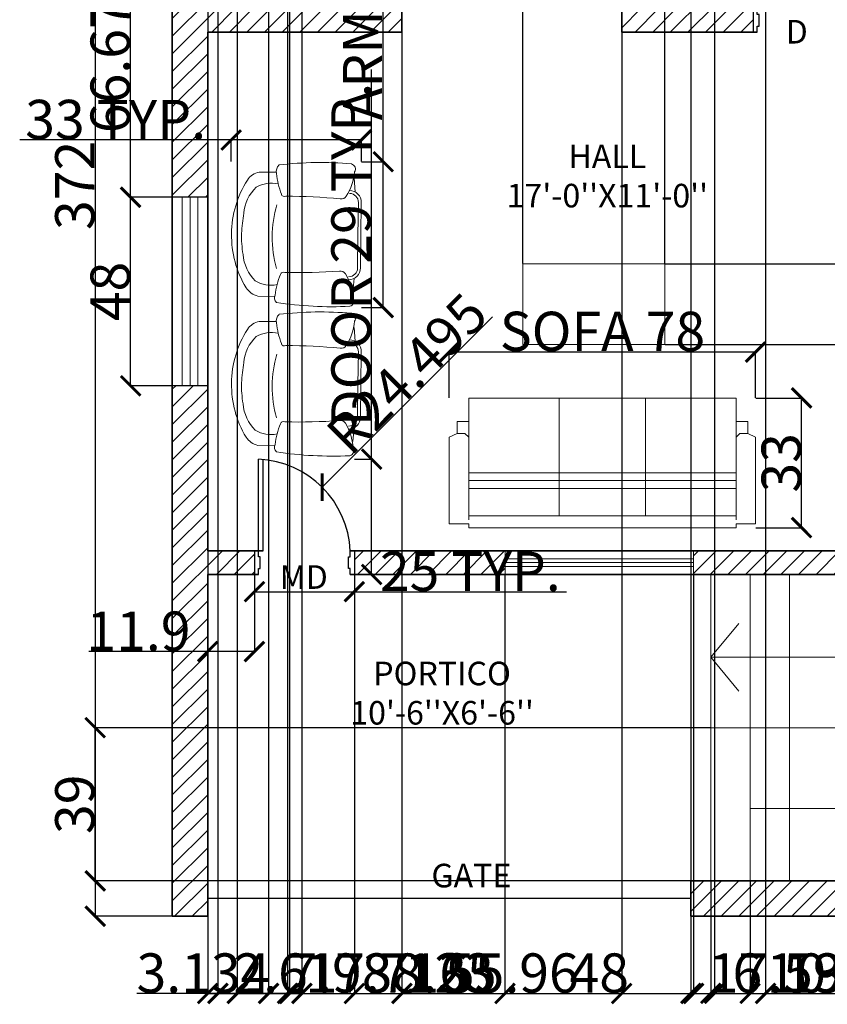
# Model space of a CAD drawing. Units: inches. Extents: x 90933 to 91345, y 21207 to 21646.
# Tile 1 of 4: x 90989 to 91195, y 21207 to 21458. Entities that reach past the tile are written whole.
import ezdxf

# ---------------------------------------------------------------- set-up
doc = ezdxf.new("R2010")
doc.units = ezdxf.units.IN
for name, color, linetype, lineweight in [('A-ANNO-DIMS', 2, 'Continuous', 18), ('A-ANNO-TEXT', 7, 'Continuous', 18), ('A-AREA-IDEN', 7, 'Continuous', 25), ('A-WALL-PATT', 8, 'Continuous', 13), ('B-FURNITURE', 9, 'Continuous', 18), ('Doors', 34, 'Continuous', 25), ('Steps', 50, 'Continuous', 18), ('Walls', 7, 'Continuous', 35), ('Windows', 140, 'Continuous', 18)]:
    doc.layers.add(name, color=color, linetype=linetype, lineweight=lineweight)
doc.styles.get("Standard").update_dxf_attribs({"font": 'arial.ttf'})
doc.dimstyles.get("Standard").update_dxf_attribs({"dimtxt": 10, "dimasz": 5, "dimexe": 0.18, "dimexo": 0.0625, "dimgap": 0.09, "dimtad": 1, "dimdec": 1, "dimzin": 0, "dimdsep": 46, "dimlunit": 4, "dimtxsty": 'Standard', "dimblk": 'ARCHTICK', "dimcen": 0.09, "dimadec": 0, "dimazin": 0, "dimtfac": 1, "dimtdec": 1, "dimtofl": 0, "dimtmove": 0, "dimatfit": 3, "dimldrblk": 'NONE', "dimfxl": 1, "dimtolj": 1, "dimtzin": 0, "dimarcsym": 0})

# ---------------------------------------------------------------- blocks, each defined once
blk = doc.blocks.new('12PCOU13')
at = {"color": 0, "linetype": 'ByBlock'}
for p, q in [((24, 37), (24, 35)), ((23, 34), (2, 34)), ((3, -34), (3, 34)), ((10, 34), (10, -34)), ((12, 34), (12, -34)), ((14, 34), (14, -34)), ((24, 35), (23, 34)), ((27, 34), (23, 34)), ((33, 11), (3, 11)), ((33, -11), (3, -11)), ((23, -34), (2, -34)), ((27, -34), (23, -34)), ((24, -35), (23, -34)), ((24, -37), (24, -35))]:
    blk.add_line(p, q, dxfattribs=at)
blk.add_lwpolyline([(1, -39), (1, -34), (0, -34), (0, 34), (1, 34), (1, 39), (23, 39), (24, 37), (27, 37), (27, 34), (33, 34), (33, -34), (27, -34), (27, -37), (24, -37), (23, -39)], close=True, dxfattribs=at)
blk = doc.blocks.new('A$C198557BC')
for p, q in [((-0.4117, 0.5807), (-0.4097, 0.6946)), ((0.4248, 0.5712), (0.4254, 0.6851)), ((-0.2994, 0.0834), (-0.2994, 0.0852)), ((0.3012, 0.0766), (0.3012, 0.0783)), ((-0.2905, 0.0459), (-0.3822, 0.0549)), ((0, 0), (-0.2203, 0.0025)), ((0.0002, 0.02), (-0.2201, 0.0225)), ((0, 0), (0.2203, -0.0025)), ((0.0002, 0.02), (0.2205, 0.0175)), ((0.2915, 0.0393), (0.3834, 0.0462))]:
    blk.add_line(p, q)
for centre, radius, start, end in [((-0.0029, 0.1962), 0.6755, 88.91413, 121.26982), ((0.0052, 0.1888), 0.6828, 57.60493, 89.60231), ((-0.0116, 0.1353), 0.6691, 87.97145, 100.08803), ((-0.0406, -0.2707), 1.076, 79.8996, 87.1923), ((-0.2885, 0.6678), 0.1242, 121.56358, 167.53067), ((-0.1087, 0.5143), 0.2805, 94.11543, 135.13675), ((0.1307, 0.5261), 0.2631, 42.84347, 86.21861), ((0.3036, 0.661), 0.1242, 11.16492, 57.13201), ((-0.132, 0.6064), 0.2049, 148.9368, 191.77668), ((0.1457, 0.6033), 0.2049, 346.91891, 29.75879), ((-0.0152, -0.1978), 0.7955, 73.93972, 105.23292), ((1.9871, 0.1943), 2.4688, 171.25046, 182.77379), ((-0.4204, 0.533), 0.0491, 69.35384, 131.44148), ((-0.4978, -0.067), 0.6529, 68.98758, 81.6584), ((-0.2691, 0.5224), 0.0208, 332.44605, 75.17429), ((0.2809, 0.5161), 0.0208, 103.52131, 206.24954), ((0.4962, -0.0783), 0.6529, 97.03719, 109.70801), ((0.4268, 0.5037), 0.0668, 46.11764, 99.16123), ((-1.9034, 0.2728), 2.3929, 354.99182, 6.69659), ((3.0866, 0.4124), 3.3387, 178.2785, 184.60096), ((-3.0764, 0.4826), 3.3387, 354.09463, 0.41709), ((-0.2813, 0.1392), 0.0403, 300.81783, 7.8066), ((0.2844, 0.1327), 0.0403, 170.889, 237.87776), ((-0.4437, 0.0838), 0.0362, 194.45648, 300.66989), ((-0.4522, 0.4253), 0.3736, 274.13358, 300.83861), ((-0.2194, 0.0825), 0.08, 179.3478, 269.3478), ((-0.2194, 0.0825), 0.06, 179.3478, 269.3478), ((0.2212, 0.0775), 0.08, 269.3478, 359.3478), ((0.2212, 0.0775), 0.06, 269.3478, 359.3478), ((0.4617, 0.4149), 0.3736, 237.85698, 264.56202), ((0.4455, 0.0737), 0.0362, 238.0257, 344.23911)]:
    blk.add_arc(centre, radius, start, end)
blk = doc.blocks.new('AP0B05')
for p, q in [((35, 100), (35, 880)), ((75, 100), (75, 878.9))]:
    blk.add_line(p, q)
for points in [[(0, 100), (0, -100), (35, -100), (35, -50), (50, -50), (50, 50), (35, 50), (35, 100)], [(850, 100), (850, -100), (815, -100), (815, -50), (800, -50), (800, 50), (815, 50), (815, 100)]]:
    blk.add_lwpolyline(points, close=True)
blk.add_lwpolyline([(35, 100), (75, 100)])
blk.add_arc((-2.4, 62.6), 818.3, 2.62122, 87.37878)
blk = doc.blocks.new('_ArchTick')
at = {"color": 0, "linetype": 'ByBlock', "const_width": 0.15}
blk.add_lwpolyline([(-0.5, -0.5), (0.5, 0.5)], dxfattribs=at)
blk = doc.blocks.new('*D20')
at = {"layer": 'A-ANNO-DIMS', "color": 0, "lineweight": -2, "transparency": 16777216}
for p, q in [((91078.84, 21345.95), (91078.84, 21445.1)), ((91074.51, 21345.95), (91079.02, 21345.95)), ((91078.84, 21316.62), (91078.84, 21345.95)), ((91074.51, 21316.62), (91079.02, 21316.62))]:
    blk.add_line(p, q, dxfattribs=at)
at = {"layer": 'Defpoints', "color": 0, "transparency": 16777216}
for p in [(91074.44, 21345.95), (91078.84, 21345.95), (91074.44, 21316.62)]:
    blk.add_point(p, dxfattribs=at)
at = {"layer": 'A-ANNO-DIMS', "color": 0, "lineweight": -2, "transparency": 16777216, "xscale": 5, "yscale": 5, "zscale": 5}
for p, rotation in [((91078.84, 21345.95), 90), ((91078.84, 21316.62), 270)]:
    blk.add_blockref('_ArchTick', p, dxfattribs=dict(at, rotation=rotation))
at = {"layer": 'A-ANNO-DIMS', "color": 0, "transparency": 16777216, "insert": (91073.58, 21398.03), "char_height": 10, "attachment_point": 5, "rotation": 90}
blk.add_mtext('\\A1;DOOR 29 TYP.', dxfattribs=at)
blk = doc.blocks.new('_None')
blk = doc.blocks.new('*D21')
at = {"layer": 'A-ANNO-DIMS', "color": 0, "lineweight": -2, "transparency": 16777216}
for p, q in [((91049, 21316.55), (91049, 21312.04)), ((91074.44, 21316.55), (91074.44, 21312.04)), ((91049, 21312.22), (91074.44, 21312.22)), ((91074.44, 21312.22), (91128.47, 21312.22))]:
    blk.add_line(p, q, dxfattribs=at)
at = {"layer": 'Defpoints', "color": 0, "transparency": 16777216}
for p in [(91049, 21316.62), (91074.44, 21316.62), (91074.44, 21312.22)]:
    blk.add_point(p, dxfattribs=at)
at = {"layer": 'A-ANNO-DIMS', "color": 0, "lineweight": -2, "transparency": 16777216, "xscale": 5, "yscale": 5, "zscale": 5, "rotation": 180}
blk.add_blockref('_ArchTick', (91049, 21312.22), dxfattribs=at)
at = {"layer": 'A-ANNO-DIMS', "color": 0, "lineweight": -2, "transparency": 16777216, "xscale": 5, "yscale": 5, "zscale": 5}
blk.add_blockref('_ArchTick', (91074.44, 21312.22), dxfattribs=at)
at = {"layer": 'A-ANNO-DIMS', "color": 0, "transparency": 16777216, "insert": (91103.96, 21317.41), "char_height": 10, "attachment_point": 5}
blk.add_mtext('\\A1;25 TYP.', dxfattribs=at)
blk = doc.blocks.new('*D24')
at = {"layer": 'A-ANNO-DIMS', "color": 0, "lineweight": -2, "transparency": 16777216}
for p, q in [((91081.79, 21421.63), (91081.79, 21554.45)), ((91076.29, 21421.63), (91081.97, 21421.63)), ((91081.79, 21384.54), (91081.79, 21421.63)), ((91076.29, 21384.54), (91081.97, 21384.54))]:
    blk.add_line(p, q, dxfattribs=at)
at = {"layer": 'Defpoints', "color": 0, "transparency": 16777216}
for p in [(91076.22, 21421.63), (91081.79, 21421.63), (91076.22, 21384.54)]:
    blk.add_point(p, dxfattribs=at)
at = {"layer": 'A-ANNO-DIMS', "color": 0, "lineweight": -2, "transparency": 16777216, "xscale": 5, "yscale": 5, "zscale": 5}
for p, rotation in [((91081.79, 21421.63), 90), ((91081.79, 21384.54), 270)]:
    blk.add_blockref('_ArchTick', p, dxfattribs=dict(at, rotation=rotation))
at = {"layer": 'A-ANNO-DIMS', "color": 0, "transparency": 16777216, "insert": (91076.52, 21490.54), "char_height": 10, "attachment_point": 5, "rotation": 90}
blk.add_mtext('\\A1;ARMCHAIR 37 TYP.', dxfattribs=at)
blk = doc.blocks.new('*D25')
at = {"layer": 'A-ANNO-DIMS', "color": 0, "lineweight": -2, "transparency": 16777216}
for p, q in [((91043.09, 21427.19), (90989.24, 21427.19)), ((91043.09, 21421.69), (91043.09, 21427.37)), ((91076.22, 21427.19), (91043.09, 21427.19)), ((91076.22, 21421.69), (91076.22, 21427.37))]:
    blk.add_line(p, q, dxfattribs=at)
at = {"layer": 'Defpoints', "color": 0, "transparency": 16777216}
for p in [(91043.09, 21427.19), (91043.09, 21421.63), (91076.22, 21421.63)]:
    blk.add_point(p, dxfattribs=at)
at = {"layer": 'A-ANNO-DIMS', "color": 0, "lineweight": -2, "transparency": 16777216, "xscale": 5, "yscale": 5, "zscale": 5, "rotation": 180}
blk.add_blockref('_ArchTick', (91043.09, 21427.19), dxfattribs=at)
at = {"layer": 'A-ANNO-DIMS', "color": 0, "lineweight": -2, "transparency": 16777216, "xscale": 5, "yscale": 5, "zscale": 5}
blk.add_blockref('_ArchTick', (91076.22, 21427.19), dxfattribs=at)
at = {"layer": 'A-ANNO-DIMS', "color": 0, "transparency": 16777216, "insert": (91013.67, 21432.39), "char_height": 10, "attachment_point": 5}
blk.add_mtext('\\A1;33 TYP.', dxfattribs=at)
blk = doc.blocks.new('*D28')
at = {"layer": 'A-ANNO-DIMS', "color": 0, "lineweight": -2, "transparency": 16777216}
for p, q in [((91098.6, 21361.57), (91098.6, 21373.39)), ((91176.6, 21373.21), (91098.6, 21373.21)), ((91176.6, 21361.57), (91176.6, 21373.39))]:
    blk.add_line(p, q, dxfattribs=at)
at = {"layer": 'Defpoints', "color": 0, "transparency": 16777216}
for p in [(91098.6, 21373.21), (91098.6, 21361.51), (91176.6, 21361.51)]:
    blk.add_point(p, dxfattribs=at)
at = {"layer": 'A-ANNO-DIMS', "color": 0, "lineweight": -2, "transparency": 16777216, "xscale": 5, "yscale": 5, "zscale": 5, "rotation": 180}
blk.add_blockref('_ArchTick', (91098.6, 21373.21), dxfattribs=at)
at = {"layer": 'A-ANNO-DIMS', "color": 0, "lineweight": -2, "transparency": 16777216, "xscale": 5, "yscale": 5, "zscale": 5}
blk.add_blockref('_ArchTick', (91176.6, 21373.21), dxfattribs=at)
at = {"layer": 'A-ANNO-DIMS', "color": 0, "transparency": 16777216, "insert": (91137.6, 21378.47), "char_height": 10, "attachment_point": 5}
blk.add_mtext('\\A1;SOFA 78', dxfattribs=at)
blk = doc.blocks.new('*D29')
at = {"layer": 'A-ANNO-DIMS', "color": 0, "lineweight": -2, "transparency": 16777216}
for p, q in [((91176.66, 21361.51), (91188.48, 21361.51)), ((91188.3, 21328.51), (91188.3, 21361.51)), ((91176.66, 21328.51), (91188.48, 21328.51))]:
    blk.add_line(p, q, dxfattribs=at)
at = {"layer": 'Defpoints', "color": 0, "transparency": 16777216}
for p in [(91176.6, 21361.51), (91188.3, 21361.51), (91176.6, 21328.51)]:
    blk.add_point(p, dxfattribs=at)
at = {"layer": 'A-ANNO-DIMS', "color": 0, "lineweight": -2, "transparency": 16777216, "xscale": 5, "yscale": 5, "zscale": 5}
for p, rotation in [((91188.3, 21361.51), 90), ((91188.3, 21328.51), 270)]:
    blk.add_blockref('_ArchTick', p, dxfattribs=dict(at, rotation=rotation))
at = {"layer": 'A-ANNO-DIMS', "color": 0, "transparency": 16777216, "insert": (91183.1, 21345.01), "char_height": 10, "attachment_point": 5, "rotation": 90}
blk.add_mtext('\\A1;33', dxfattribs=at)
blk = doc.blocks.new('*D38')
at = {"layer": 'A-ANNO-DIMS', "color": 0, "lineweight": -2, "transparency": 16777216}
for p, q in [((91037.1, 21229.55), (91037.1, 21209.81)), ((91160.1, 21229.55), (91160.1, 21209.81)), ((91037.1, 21209.99), (91160.1, 21209.99))]:
    blk.add_line(p, q, dxfattribs=at)
at = {"layer": 'Defpoints', "color": 0, "transparency": 16777216}
for p in [(91037.1, 21229.62), (91160.1, 21229.62), (91160.1, 21209.99)]:
    blk.add_point(p, dxfattribs=at)
at = {"layer": 'A-ANNO-DIMS', "color": 0, "lineweight": -2, "transparency": 16777216, "xscale": 5, "yscale": 5, "zscale": 5, "rotation": 180}
blk.add_blockref('_ArchTick', (91037.1, 21209.99), dxfattribs=at)
at = {"layer": 'A-ANNO-DIMS', "color": 0, "lineweight": -2, "transparency": 16777216, "xscale": 5, "yscale": 5, "zscale": 5}
blk.add_blockref('_ArchTick', (91160.1, 21209.99), dxfattribs=at)
at = {"layer": 'A-ANNO-DIMS', "color": 0, "transparency": 16777216, "insert": (91098.6, 21215.18), "char_height": 10, "attachment_point": 5}
blk.add_mtext('\\A1;123', dxfattribs=at)
blk = doc.blocks.new('*D41')
at = {"layer": 'A-ANNO-DIMS', "color": 0, "lineweight": -2, "transparency": 16777216}
for p, q in [((91166.1, 21592.55), (91166.1, 21209.81)), ((91179.14, 21592.55), (91179.14, 21209.81)), ((91166.1, 21209.99), (91179.14, 21209.99)), ((91179.14, 21209.99), (91224.86, 21209.99))]:
    blk.add_line(p, q, dxfattribs=at)
at = {"layer": 'Defpoints', "color": 0, "transparency": 16777216}
for p in [(91166.1, 21592.62), (91179.14, 21592.62), (91179.14, 21209.99)]:
    blk.add_point(p, dxfattribs=at)
at = {"layer": 'A-ANNO-DIMS', "color": 0, "lineweight": -2, "transparency": 16777216, "xscale": 5, "yscale": 5, "zscale": 5, "rotation": 180}
blk.add_blockref('_ArchTick', (91166.1, 21209.99), dxfattribs=at)
at = {"layer": 'A-ANNO-DIMS', "color": 0, "lineweight": -2, "transparency": 16777216, "xscale": 5, "yscale": 5, "zscale": 5}
blk.add_blockref('_ArchTick', (91179.14, 21209.99), dxfattribs=at)
at = {"layer": 'A-ANNO-DIMS', "color": 0, "transparency": 16777216, "insert": (91204.5, 21215.18), "char_height": 10, "attachment_point": 5}
blk.add_mtext('\\A1;13.044', dxfattribs=at)
blk = doc.blocks.new('*D43')
at = {"layer": 'A-ANNO-DIMS', "color": 0, "lineweight": -2, "transparency": 16777216}
for p, q in [((91037.04, 21479.28), (91017.29, 21479.28)), ((91017.47, 21412.62), (91017.47, 21479.28)), ((91037.04, 21412.62), (91017.29, 21412.62))]:
    blk.add_line(p, q, dxfattribs=at)
at = {"layer": 'Defpoints', "color": 0, "transparency": 16777216}
for p in [(91017.47, 21479.28), (91037.1, 21479.28), (91037.1, 21412.62)]:
    blk.add_point(p, dxfattribs=at)
at = {"layer": 'A-ANNO-DIMS', "color": 0, "lineweight": -2, "transparency": 16777216, "xscale": 5, "yscale": 5, "zscale": 5}
for p, rotation in [((91017.47, 21479.28), 90), ((91017.47, 21412.62), 270)]:
    blk.add_blockref('_ArchTick', p, dxfattribs=dict(at, rotation=rotation))
at = {"layer": 'A-ANNO-DIMS', "color": 0, "transparency": 16777216, "insert": (91012.27, 21445.95), "char_height": 10, "attachment_point": 5, "rotation": 90}
blk.add_mtext('\\A1;66.67', dxfattribs=at)
blk = doc.blocks.new('*D44')
at = {"layer": 'A-ANNO-DIMS', "color": 0, "lineweight": -2, "transparency": 16777216}
for p, q in [((91037.04, 21412.62), (91017.29, 21412.62)), ((91017.47, 21364.62), (91017.47, 21412.62)), ((91037.04, 21364.62), (91017.29, 21364.62))]:
    blk.add_line(p, q, dxfattribs=at)
at = {"layer": 'Defpoints', "color": 0, "transparency": 16777216}
for p in [(91017.47, 21412.62), (91037.1, 21412.62), (91037.1, 21364.62)]:
    blk.add_point(p, dxfattribs=at)
at = {"layer": 'A-ANNO-DIMS', "color": 0, "lineweight": -2, "transparency": 16777216, "xscale": 5, "yscale": 5, "zscale": 5}
for p, rotation in [((91017.47, 21412.62), 90), ((91017.47, 21364.62), 270)]:
    blk.add_blockref('_ArchTick', p, dxfattribs=dict(at, rotation=rotation))
at = {"layer": 'A-ANNO-DIMS', "color": 0, "transparency": 16777216, "insert": (91012.27, 21388.62), "char_height": 10, "attachment_point": 5, "rotation": 90}
blk.add_mtext('\\A1;48', dxfattribs=at)
blk = doc.blocks.new('*D45')
at = {"layer": 'A-ANNO-DIMS', "color": 0, "lineweight": -2, "transparency": 16777216}
for p, q in [((91112.79, 21316.55), (91112.79, 21209.81)), ((91160.79, 21316.55), (91160.79, 21209.81)), ((91112.79, 21209.99), (91160.79, 21209.99))]:
    blk.add_line(p, q, dxfattribs=at)
at = {"layer": 'Defpoints', "color": 0, "transparency": 16777216}
for p in [(91112.79, 21316.62), (91160.79, 21316.62), (91160.79, 21209.99)]:
    blk.add_point(p, dxfattribs=at)
at = {"layer": 'A-ANNO-DIMS', "color": 0, "lineweight": -2, "transparency": 16777216, "xscale": 5, "yscale": 5, "zscale": 5, "rotation": 180}
blk.add_blockref('_ArchTick', (91112.79, 21209.99), dxfattribs=at)
at = {"layer": 'A-ANNO-DIMS', "color": 0, "lineweight": -2, "transparency": 16777216, "xscale": 5, "yscale": 5, "zscale": 5}
blk.add_blockref('_ArchTick', (91160.79, 21209.99), dxfattribs=at)
at = {"layer": 'A-ANNO-DIMS', "color": 0, "transparency": 16777216, "insert": (91136.79, 21215.18), "char_height": 10, "attachment_point": 5}
blk.add_mtext('\\A1;48', dxfattribs=at)
blk = doc.blocks.new('*D46')
at = {"layer": 'A-ANNO-DIMS', "color": 0, "lineweight": -2, "transparency": 16777216}
for p, q in [((91037.1, 21316.55), (91037.1, 21296.81)), ((91049, 21316.55), (91049, 21296.81)), ((91037.1, 21296.99), (91006.87, 21296.99)), ((91049, 21296.99), (91037.1, 21296.99))]:
    blk.add_line(p, q, dxfattribs=at)
at = {"layer": 'Defpoints', "color": 0, "transparency": 16777216}
for p in [(91037.1, 21316.62), (91049, 21316.62), (91037.1, 21296.99)]:
    blk.add_point(p, dxfattribs=at)
at = {"layer": 'A-ANNO-DIMS', "color": 0, "lineweight": -2, "transparency": 16777216, "xscale": 5, "yscale": 5, "zscale": 5}
for p, rotation in [((91037.1, 21296.99), 179.9999999999825), ((91049, 21296.99), 359.9999999999825)]:
    blk.add_blockref('_ArchTick', p, dxfattribs=dict(at, rotation=rotation))
at = {"layer": 'A-ANNO-DIMS', "color": 0, "transparency": 16777216, "insert": (91019.48, 21302.18), "char_height": 10, "attachment_point": 5}
blk.add_mtext('\\A1;11.9', dxfattribs=at)
blk = doc.blocks.new('*D47')
at = {"layer": 'A-ANNO-DIMS', "color": 0, "lineweight": -2, "transparency": 16777216}
for p, q in [((91074.44, 21316.55), (91074.44, 21209.81)), ((91112.79, 21316.55), (91112.79, 21209.81)), ((91074.44, 21209.99), (91112.79, 21209.99))]:
    blk.add_line(p, q, dxfattribs=at)
at = {"layer": 'Defpoints', "color": 0, "transparency": 16777216}
for p in [(91074.44, 21316.62), (91112.79, 21316.62), (91112.79, 21209.99)]:
    blk.add_point(p, dxfattribs=at)
at = {"layer": 'A-ANNO-DIMS', "color": 0, "lineweight": -2, "transparency": 16777216, "xscale": 5, "yscale": 5, "zscale": 5, "rotation": 180}
blk.add_blockref('_ArchTick', (91074.44, 21209.99), dxfattribs=at)
at = {"layer": 'A-ANNO-DIMS', "color": 0, "lineweight": -2, "transparency": 16777216, "xscale": 5, "yscale": 5, "zscale": 5}
blk.add_blockref('_ArchTick', (91112.79, 21209.99), dxfattribs=at)
at = {"layer": 'A-ANNO-DIMS', "color": 0, "transparency": 16777216, "insert": (91093.62, 21215.18), "char_height": 10, "attachment_point": 5}
blk.add_mtext('\\A1;38.35', dxfattribs=at)
blk = doc.blocks.new('*D48')
at = {"layer": 'A-ANNO-DIMS', "color": 0, "lineweight": -2, "transparency": 16777216}
for p, q in [((91086.54, 21454.55), (91086.54, 21209.81)), ((91142.5, 21454.55), (91142.5, 21209.81)), ((91086.54, 21209.99), (91142.5, 21209.99))]:
    blk.add_line(p, q, dxfattribs=at)
at = {"layer": 'Defpoints', "color": 0, "transparency": 16777216}
for p in [(91086.54, 21454.62), (91142.5, 21454.62), (91142.5, 21209.99)]:
    blk.add_point(p, dxfattribs=at)
at = {"layer": 'A-ANNO-DIMS', "color": 0, "lineweight": -2, "transparency": 16777216, "xscale": 5, "yscale": 5, "zscale": 5, "rotation": 180}
blk.add_blockref('_ArchTick', (91086.54, 21209.99), dxfattribs=at)
at = {"layer": 'A-ANNO-DIMS', "color": 0, "lineweight": -2, "transparency": 16777216, "xscale": 5, "yscale": 5, "zscale": 5}
blk.add_blockref('_ArchTick', (91142.5, 21209.99), dxfattribs=at)
at = {"layer": 'A-ANNO-DIMS', "color": 0, "transparency": 16777216, "insert": (91114.52, 21215.18), "char_height": 10, "attachment_point": 5}
blk.add_mtext('\\A1;55.96', dxfattribs=at)
blk = doc.blocks.new('*D49')
at = {"layer": 'A-ANNO-DIMS', "color": 0, "lineweight": -2, "transparency": 16777216}
for p, q in [((91160.1, 21460.55), (91160.1, 21209.81)), ((91142.5, 21454.55), (91142.5, 21209.81)), ((91142.5, 21209.99), (91160.1, 21209.99)), ((91160.1, 21209.99), (91205.85, 21209.99))]:
    blk.add_line(p, q, dxfattribs=at)
at = {"layer": 'Defpoints', "color": 0, "transparency": 16777216}
for p in [(91160.1, 21460.62), (91142.5, 21454.62), (91160.1, 21209.99)]:
    blk.add_point(p, dxfattribs=at)
at = {"layer": 'A-ANNO-DIMS', "color": 0, "lineweight": -2, "transparency": 16777216, "xscale": 5, "yscale": 5, "zscale": 5, "rotation": 180}
blk.add_blockref('_ArchTick', (91142.5, 21209.99), dxfattribs=at)
at = {"layer": 'A-ANNO-DIMS', "color": 0, "lineweight": -2, "transparency": 16777216, "xscale": 5, "yscale": 5, "zscale": 5}
blk.add_blockref('_ArchTick', (91160.1, 21209.99), dxfattribs=at)
at = {"layer": 'A-ANNO-DIMS', "color": 0, "transparency": 16777216, "insert": (91185.47, 21215.18), "char_height": 10, "attachment_point": 5}
blk.add_mtext('\\A1;17.596', dxfattribs=at)
blk = doc.blocks.new('*D53')
at = {"layer": 'A-ANNO-DIMS', "color": 0, "lineweight": -2, "transparency": 16777216}
for p, q in [((91160.1, 21460.55), (91160.1, 21209.81)), ((91166.1, 21460.55), (91166.1, 21209.81)), ((91160.1, 21209.99), (91166.1, 21209.99)), ((91166.1, 21209.99), (91177.88, 21209.99))]:
    blk.add_line(p, q, dxfattribs=at)
at = {"layer": 'Defpoints', "color": 0, "transparency": 16777216}
for p in [(91160.1, 21460.62), (91166.1, 21460.62), (91166.1, 21209.99)]:
    blk.add_point(p, dxfattribs=at)
at = {"layer": 'A-ANNO-DIMS', "color": 0, "lineweight": -2, "transparency": 16777216, "xscale": 5, "yscale": 5, "zscale": 5, "rotation": 180}
blk.add_blockref('_ArchTick', (91160.1, 21209.99), dxfattribs=at)
at = {"layer": 'A-ANNO-DIMS', "color": 0, "lineweight": -2, "transparency": 16777216, "xscale": 5, "yscale": 5, "zscale": 5}
blk.add_blockref('_ArchTick', (91166.1, 21209.99), dxfattribs=at)
at = {"layer": 'A-ANNO-DIMS', "color": 0, "transparency": 16777216, "insert": (91174.49, 21215.18), "char_height": 10, "attachment_point": 5}
blk.add_mtext('\\A1;6', dxfattribs=at)
blk = doc.blocks.new('*D55')
at = {"layer": 'A-ANNO-DIMS', "color": 0, "lineweight": -2, "transparency": 16777216}
for p, q in [((91165.18, 21238.55), (91165.18, 21209.81)), ((91175.18, 21238.55), (91175.18, 21209.81)), ((91165.18, 21209.99), (91175.18, 21209.99)), ((91175.18, 21209.99), (91193.71, 21209.99))]:
    blk.add_line(p, q, dxfattribs=at)
at = {"layer": 'Defpoints', "color": 0, "transparency": 16777216}
for p in [(91165.18, 21238.62), (91175.18, 21238.62), (91175.18, 21209.99)]:
    blk.add_point(p, dxfattribs=at)
at = {"layer": 'A-ANNO-DIMS', "color": 0, "lineweight": -2, "transparency": 16777216, "xscale": 5, "yscale": 5, "zscale": 5, "rotation": 180}
blk.add_blockref('_ArchTick', (91165.18, 21209.99), dxfattribs=at)
at = {"layer": 'A-ANNO-DIMS', "color": 0, "lineweight": -2, "transparency": 16777216, "xscale": 5, "yscale": 5, "zscale": 5}
blk.add_blockref('_ArchTick', (91175.18, 21209.99), dxfattribs=at)
at = {"layer": 'A-ANNO-DIMS', "color": 0, "transparency": 16777216, "insert": (91186.94, 21215.18), "char_height": 10, "attachment_point": 5}
blk.add_mtext('\\A1;10', dxfattribs=at)
blk = doc.blocks.new('*D57')
at = {"layer": 'A-ANNO-DIMS', "color": 0, "lineweight": -2, "transparency": 16777216}
for p, q in [((91165.11, 21277.62), (91008.29, 21277.62)), ((91008.47, 21238.62), (91008.47, 21277.62)), ((91165.11, 21238.62), (91008.29, 21238.62))]:
    blk.add_line(p, q, dxfattribs=at)
at = {"layer": 'Defpoints', "color": 0, "transparency": 16777216}
for p in [(91008.47, 21277.62), (91165.18, 21277.62), (91165.18, 21238.62)]:
    blk.add_point(p, dxfattribs=at)
at = {"layer": 'A-ANNO-DIMS', "color": 0, "lineweight": -2, "transparency": 16777216, "xscale": 5, "yscale": 5, "zscale": 5}
for p, rotation in [((91008.47, 21277.62), 90), ((91008.47, 21238.62), 270)]:
    blk.add_blockref('_ArchTick', p, dxfattribs=dict(at, rotation=rotation))
at = {"layer": 'A-ANNO-DIMS', "color": 0, "transparency": 16777216, "insert": (91003.27, 21258.12), "char_height": 10, "attachment_point": 5, "rotation": 90}
blk.add_mtext('\\A1;39', dxfattribs=at)
blk = doc.blocks.new('*D58')
at = {"layer": 'A-ANNO-DIMS', "color": 0, "lineweight": -2, "transparency": 16777216}
for p, q in [((91039.71, 21517.79), (91039.71, 21209.81)), ((91057.43, 21517.79), (91057.43, 21209.81)), ((91039.71, 21209.99), (91057.43, 21209.99)), ((91057.43, 21209.99), (91103.17, 21209.99))]:
    blk.add_line(p, q, dxfattribs=at)
at = {"layer": 'Defpoints', "color": 0, "transparency": 16777216}
for p in [(91039.71, 21517.85), (91057.43, 21517.85), (91057.43, 21209.99)]:
    blk.add_point(p, dxfattribs=at)
at = {"layer": 'A-ANNO-DIMS', "color": 0, "lineweight": -2, "transparency": 16777216, "xscale": 5, "yscale": 5, "zscale": 5, "rotation": 180}
blk.add_blockref('_ArchTick', (91039.71, 21209.99), dxfattribs=at)
at = {"layer": 'A-ANNO-DIMS', "color": 0, "lineweight": -2, "transparency": 16777216, "xscale": 5, "yscale": 5, "zscale": 5}
blk.add_blockref('_ArchTick', (91057.43, 21209.99), dxfattribs=at)
at = {"layer": 'A-ANNO-DIMS', "color": 0, "transparency": 16777216, "insert": (91082.8, 21215.18), "char_height": 10, "attachment_point": 5}
blk.add_mtext('\\A1;17.716', dxfattribs=at)
blk = doc.blocks.new('*D60')
at = {"layer": 'A-ANNO-DIMS', "color": 0, "lineweight": -2, "transparency": 16777216}
for p, q in [((91117.31, 21395.74), (91117.31, 21621.43)), ((91117.31, 21621.25), (91153.51, 21621.25)), ((91153.51, 21395.74), (91153.51, 21621.43))]:
    blk.add_line(p, q, dxfattribs=at)
at = {"layer": 'Defpoints', "color": 0, "transparency": 16777216}
for p in [(91153.51, 21621.25), (91117.31, 21395.68), (91153.51, 21395.68)]:
    blk.add_point(p, dxfattribs=at)
at = {"layer": 'A-ANNO-DIMS', "color": 0, "lineweight": -2, "transparency": 16777216, "xscale": 5, "yscale": 5, "zscale": 5, "rotation": 180}
blk.add_blockref('_ArchTick', (91117.31, 21621.25), dxfattribs=at)
at = {"layer": 'A-ANNO-DIMS', "color": 0, "lineweight": -2, "transparency": 16777216, "xscale": 5, "yscale": 5, "zscale": 5}
blk.add_blockref('_ArchTick', (91153.51, 21621.25), dxfattribs=at)
at = {"layer": 'A-ANNO-DIMS', "color": 0, "transparency": 16777216, "insert": (91135.41, 21626.44), "char_height": 10, "attachment_point": 5}
blk.add_mtext('\\A1;36.2', dxfattribs=at)
blk = doc.blocks.new('*D61')
at = {"layer": 'A-ANNO-DIMS', "color": 0, "lineweight": -2, "transparency": 16777216}
for p, q in [((91326.73, 21395.68), (91326.73, 21442.44)), ((91153.57, 21395.68), (91326.91, 21395.68)), ((91326.73, 21375.15), (91326.73, 21395.68)), ((91153.57, 21375.15), (91326.91, 21375.15))]:
    blk.add_line(p, q, dxfattribs=at)
at = {"layer": 'Defpoints', "color": 0, "transparency": 16777216}
for p in [(91153.51, 21395.68), (91326.73, 21395.68), (91153.51, 21375.15)]:
    blk.add_point(p, dxfattribs=at)
at = {"layer": 'A-ANNO-DIMS', "color": 0, "lineweight": -2, "transparency": 16777216, "xscale": 5, "yscale": 5, "zscale": 5}
for p, rotation in [((91326.73, 21395.68), 90), ((91326.73, 21375.15), 270)]:
    blk.add_blockref('_ArchTick', p, dxfattribs=dict(at, rotation=rotation))
at = {"layer": 'A-ANNO-DIMS', "color": 0, "transparency": 16777216, "insert": (91321.53, 21421.56), "char_height": 10, "attachment_point": 5, "rotation": 90}
blk.add_mtext('\\A1;20.532', dxfattribs=at)
blk = doc.blocks.new('*D65')
at = {"layer": 'A-ANNO-DIMS', "color": 0, "lineweight": -2, "transparency": 16777216}
for p, q in [((91028.04, 21601.62), (91008.29, 21601.62)), ((91008.47, 21601.62), (91008.47, 21229.62)), ((91028.04, 21229.62), (91008.29, 21229.62))]:
    blk.add_line(p, q, dxfattribs=at)
at = {"layer": 'Defpoints', "color": 0, "transparency": 16777216}
for p in [(91028.1, 21601.62), (91008.47, 21229.62), (91028.1, 21229.62)]:
    blk.add_point(p, dxfattribs=at)
at = {"layer": 'A-ANNO-DIMS', "color": 0, "lineweight": -2, "transparency": 16777216, "xscale": 5, "yscale": 5, "zscale": 5}
for p, rotation in [((91008.47, 21601.62), 90), ((91008.47, 21229.62), 270)]:
    blk.add_blockref('_ArchTick', p, dxfattribs=dict(at, rotation=rotation))
at = {"layer": 'A-ANNO-DIMS', "color": 0, "transparency": 16777216, "insert": (91003.27, 21415.62), "char_height": 10, "attachment_point": 5, "rotation": 90}
blk.add_mtext('\\A1;372', dxfattribs=at)
blk = doc.blocks.new('*D71')
at = {"layer": 'A-ANNO-DIMS', "color": 0, "lineweight": -2, "transparency": 16777216}
for p, q in [((91044.61, 21522.95), (91044.61, 21209.81)), ((91052.59, 21522.95), (91052.59, 21209.81)), ((91044.61, 21209.99), (91052.59, 21209.99)), ((91052.59, 21209.99), (91083.68, 21209.99))]:
    blk.add_line(p, q, dxfattribs=at)
at = {"layer": 'Defpoints', "color": 0, "transparency": 16777216}
for p in [(91044.61, 21523.01), (91052.59, 21523.01), (91052.59, 21209.99)]:
    blk.add_point(p, dxfattribs=at)
at = {"layer": 'A-ANNO-DIMS', "color": 0, "lineweight": -2, "transparency": 16777216, "xscale": 5, "yscale": 5, "zscale": 5, "rotation": 180}
blk.add_blockref('_ArchTick', (91044.61, 21209.99), dxfattribs=at)
at = {"layer": 'A-ANNO-DIMS', "color": 0, "lineweight": -2, "transparency": 16777216, "xscale": 5, "yscale": 5, "zscale": 5}
blk.add_blockref('_ArchTick', (91052.59, 21209.99), dxfattribs=at)
at = {"layer": 'A-ANNO-DIMS', "color": 0, "transparency": 16777216, "insert": (91070.64, 21215.18), "char_height": 10, "attachment_point": 5}
blk.add_mtext('\\A1;7.98', dxfattribs=at)
blk = doc.blocks.new('*D73')
at = {"layer": 'A-ANNO-DIMS', "color": 0, "lineweight": -2, "transparency": 16777216}
for p, q in [((91039.71, 21517.79), (91039.71, 21209.81)), ((91037.1, 21515.22), (91037.1, 21209.81)), ((91037.1, 21209.99), (91039.71, 21209.99)), ((91039.71, 21209.99), (91069.11, 21209.99))]:
    blk.add_line(p, q, dxfattribs=at)
at = {"layer": 'Defpoints', "color": 0, "transparency": 16777216}
for p in [(91039.71, 21517.85), (91037.1, 21515.28), (91039.71, 21209.99)]:
    blk.add_point(p, dxfattribs=at)
at = {"layer": 'A-ANNO-DIMS', "color": 0, "lineweight": -2, "transparency": 16777216, "xscale": 5, "yscale": 5, "zscale": 5, "rotation": 180}
blk.add_blockref('_ArchTick', (91037.1, 21209.99), dxfattribs=at)
at = {"layer": 'A-ANNO-DIMS', "color": 0, "lineweight": -2, "transparency": 16777216, "xscale": 5, "yscale": 5, "zscale": 5}
blk.add_blockref('_ArchTick', (91039.71, 21209.99), dxfattribs=at)
at = {"layer": 'A-ANNO-DIMS', "color": 0, "transparency": 16777216, "insert": (91056.91, 21215.18), "char_height": 10, "attachment_point": 5}
blk.add_mtext('\\A1;2.61', dxfattribs=at)
blk = doc.blocks.new('*D74')
at = {"layer": 'A-ANNO-DIMS', "color": 0, "lineweight": -2, "transparency": 16777216}
for p, q in [((91057.97, 21477.81), (91057.97, 21209.81)), ((91061.1, 21460.55), (91061.1, 21209.81)), ((91057.97, 21209.99), (91019.09, 21209.99)), ((91061.1, 21209.99), (91057.97, 21209.99))]:
    blk.add_line(p, q, dxfattribs=at)
at = {"layer": 'Defpoints', "color": 0, "transparency": 16777216}
for p in [(91057.97, 21477.87), (91061.1, 21460.62), (91057.97, 21209.99)]:
    blk.add_point(p, dxfattribs=at)
at = {"layer": 'A-ANNO-DIMS', "color": 0, "lineweight": -2, "transparency": 16777216, "xscale": 5, "yscale": 5, "zscale": 5, "rotation": 180}
blk.add_blockref('_ArchTick', (91057.97, 21209.99), dxfattribs=at)
at = {"layer": 'A-ANNO-DIMS', "color": 0, "lineweight": -2, "transparency": 16777216, "xscale": 5, "yscale": 5, "zscale": 5}
blk.add_blockref('_ArchTick', (91061.1, 21209.99), dxfattribs=at)
at = {"layer": 'A-ANNO-DIMS', "color": 0, "transparency": 16777216, "insert": (91036.03, 21215.18), "char_height": 10, "attachment_point": 5}
blk.add_mtext('\\A1;3.134', dxfattribs=at)
blk = doc.blocks.new('*D80')
at = {"layer": 'A-ANNO-DIMS', "color": 0, "lineweight": -2, "transparency": 16777216}
for p, q in [((91109.62, 21382.18), (91066.25, 21338.8)), ((91048.84, 21321.48), (91049.02, 21321.48)), ((91048.93, 21321.39), (91048.93, 21321.57))]:
    blk.add_line(p, q, dxfattribs=at)
at = {"layer": 'Defpoints', "color": 0, "transparency": 16777216}
for p in [(91066.25, 21338.8), (91048.93, 21321.48)]:
    blk.add_point(p, dxfattribs=at)
at = {"layer": 'A-ANNO-DIMS', "color": 0, "lineweight": -2, "transparency": 16777216, "xscale": 5, "yscale": 5, "zscale": 5, "rotation": 225.00088820097}
blk.add_blockref('_ArchTick', (91066.25, 21338.8), dxfattribs=at)
at = {"layer": 'A-ANNO-DIMS', "color": 0, "transparency": 16777216, "insert": (91087.8, 21367.7), "char_height": 10, "attachment_point": 5, "rotation": 45.0009}
blk.add_mtext('\\A1;R24.495', dxfattribs=at)

msp = doc.modelspace()

# ---------------------------------------------------------------- hatches: boundary and pattern name
at = {"layer": 'A-WALL-PATT', "transparency": 33554585}
h = msp.add_hatch(dxfattribs=at)
h.set_pattern_fill('ANSI31', color=256)
h.paths.add_polyline_path([(91179.1445, 21601.6157), (91028.1004, 21601.6157), (91028.1004, 21515.2814), (91037.1004, 21515.2814), (91037.1004, 21592.6157), (91160.1004, 21592.6157), (91160.1004, 21460.6157), (91142.5048, 21460.6157), (91142.5048, 21454.6157), (91175.976, 21454.6157), (91175.976, 21460.6157), (91166.1004, 21460.6157), (91166.1004, 21592.6157), (91179.1445, 21592.6157)])
h.paths.add_polyline_path([(91307.1004, 21601.6157), (91215.1445, 21601.6157), (91215.1445, 21592.6157), (91298.1004, 21592.6157), (91298.1004, 21460.6157), (91272.1605, 21460.6157), (91272.1605, 21454.6157), (91298.1004, 21454.6157), (91298.1004, 21384.4519), (91307.1004, 21384.4519)])
h.paths.add_polyline_path([(91037.1004, 21454.6157), (91086.5447, 21454.6157), (91086.5447, 21460.6157), (91037.1004, 21460.6157), (91037.1004, 21479.2814), (91028.1004, 21479.2814), (91028.1004, 21412.6157), (91037.1004, 21412.6157)])
h.paths.add_polyline_path([(91307.1004, 21348.4519), (91298.1004, 21348.4519), (91298.1004, 21322.6157), (91244.1004, 21322.6157), (91244.1004, 21454.6157), (91246.6116, 21454.6157), (91246.6116, 21460.6157), (91201.4342, 21460.6157), (91201.4342, 21454.6157), (91238.1004, 21454.6157), (91238.1004, 21322.6157), (91160.7949, 21322.6157), (91160.7949, 21316.6157), (91298.1004, 21316.6157), (91298.1004, 21238.6157), (91160.1004, 21238.6157), (91160.1004, 21229.6157), (91307.1004, 21229.6157)])
h.paths.add_polyline_path([(91037.1004, 21316.6157), (91049.0004, 21316.6157), (91049.0004, 21322.6157), (91037.1004, 21322.6157), (91037.1004, 21364.6157), (91028.1004, 21364.6157), (91028.1004, 21229.6157), (91037.1004, 21229.6157)])
h.paths.add_polyline_path([(91112.7949, 21322.6157), (91074.4445, 21322.6157), (91074.4445, 21316.6157), (91112.7949, 21316.6157)])

# ---------------------------------------------------------------- linework, layer by layer
at = {"layer": 'B-FURNITURE'}
msp.add_lwpolyline([(91117.3093, 21395.6809), (91153.5083, 21395.6809), (91153.5083, 21375.1486), (91117.3093, 21375.1486)], close=True, dxfattribs=at)
at = {"layer": 'Doors'}
msp.add_line((91160.1004, 21234.1157), (91037.1004, 21234.1157), dxfattribs=at)
at = {"layer": 'Steps'}
for p, q in [((91165.1761, 21238.6157), (91165.1761, 21316.6157)), ((91175.1761, 21238.6157), (91175.1761, 21316.6157)), ((91185.1761, 21238.6157), (91185.1761, 21316.6157)), ((91165.1761, 21277.6157), (91265.1761, 21277.6157))]:
    msp.add_line(p, q, dxfattribs=at)
for points in [[(91172.3051, 21286.9116), (91165.1761, 21295.5267), (91172.3051, 21304.1418)], [(91175.1761, 21257.0619), (91274.1452, 21257.0619), (91274.1452, 21295.5267), (91165.1761, 21295.5267)]]:
    msp.add_lwpolyline(points, dxfattribs=at)
at = {"layer": 'Walls'}
for p, q in [((91028.1004, 21601.6157), (91028.1004, 21229.6157)), ((91086.5447, 21460.6157), (91086.5447, 21454.6157)), ((91142.5048, 21460.6157), (91142.5048, 21454.6157)), ((91037.1004, 21454.6157), (91086.5447, 21454.6157)), ((91037.1004, 21454.6157), (91037.1004, 21322.6157)), ((91142.5048, 21454.6157), (91177.0243, 21454.6157)), ((91037.1004, 21322.6157), (91051.2454, 21322.6157)), ((91073.3962, 21322.6157), (91238.1004, 21322.6157)), ((91037.1004, 21316.6157), (91050.0481, 21316.6157)), ((91037.1004, 21316.6157), (91037.1004, 21229.6157)), ((91073.3968, 21316.6157), (91298.1004, 21316.6157)), ((91160.1004, 21238.6157), (91298.1004, 21238.6157)), ((91160.1004, 21238.6157), (91160.1004, 21229.6157)), ((91028.1004, 21229.6157), (91037.1004, 21229.6157)), ((91160.1004, 21229.6157), (91307.1004, 21229.6157))]:
    msp.add_line(p, q, dxfattribs=at)
at = {"layer": 'Windows'}
for p, q in [((91030.6004, 21364.6157), (91030.6004, 21412.6157)), ((91032.6004, 21364.6157), (91032.6004, 21412.6157)), ((91034.6004, 21364.6157), (91034.6004, 21412.6157)), ((91112.7949, 21320.6157), (91160.7949, 21320.6157)), ((91112.7949, 21319.6157), (91160.7949, 21319.6157)), ((91112.7949, 21318.6157), (91160.7949, 21318.6157))]:
    msp.add_line(p, q, dxfattribs=at)
for points in [[(91028.1004, 21364.6157), (91028.1004, 21412.6157), (91037.1004, 21412.6157), (91037.1004, 21364.6157)], [(91112.7949, 21322.6157), (91160.7949, 21322.6157), (91160.7949, 21316.6157), (91112.7949, 21316.6157)]]:
    msp.add_lwpolyline(points, close=True, dxfattribs=at)

# ---------------------------------------------------------------- block references
at = {"layer": 'B-FURNITURE', "xscale": 37.78817884483897, "yscale": 37.78817884483897, "zscale": 37.78817884483897, "rotation": 90}
for p in [(91076.1198, 21402.9386), (91076.1198, 21364.9256)]:
    msp.add_blockref('A$C198557BC', p, dxfattribs=at)
at = {"layer": 'B-FURNITURE', "rotation": 90}
msp.add_blockref('12PCOU13', (91137.6004, 21328.5106), dxfattribs=at)
at = {"layer": 'Doors'}
for p, xscale, yscale, zscale in [((91175.976, 21457.6107), 0.0299507821919959, 0.0299507821919959, 0.0299507821919959), ((91049.0004, 21319.6091), 0.0299343301886494, 0.0299343301886494, 0.0299343301886494)]:
    msp.add_blockref('AP0B05', p, dxfattribs=dict(at, xscale=xscale, yscale=yscale, zscale=zscale))

# ---------------------------------------------------------------- texts
at = {"layer": 'A-ANNO-TEXT'}
for s, p in [('D', (91184.2419, 21451.72)), ('MD', (91055.4088, 21312.9469)), ('GATE', (91094.0664, 21236.9782))]:
    msp.add_text(s, height=6, dxfattribs=at).set_placement(p)
at = {"layer": 'A-AREA-IDEN', "char_height": 6, "attachment_point": 1}
for s, insert in [("\\pxqc;HALL\\P17'-0''X11'-0''", (91115.754, 21426.0143)), ("\\pxqc;PORTICO\\P10'-6''X6'-6''", (91073.6792, 21294.4061))]:
    msp.add_mtext_dynamic_manual_height_columns(s, width=46.179351, gutter_width=12.5, heights=[0], dxfattribs=dict(at, insert=insert))

# ---------------------------------------------------------------- dimensions: what is measured, and where the dimension line sits
at = {"layer": 'A-ANNO-DIMS'}
for base, p1, p2, override, picture, middle in [((91153.5083, 21621.2457), (91117.3093, 21395.6809), (91153.5083, 21395.6809), {"dimdec": 1, "dimlfac": 1, "dimrnd": 0, "dimzin": 0, "dimdsep": 46, "dimlunit": 2}, '*D60', (91135.4088, 21626.4448)), ((91179.1445, 21209.9857), (91166.1004, 21592.6157), (91179.1445, 21592.6157), {"dimdec": 3, "dimlfac": 1, "dimrnd": 0, "dimzin": 0, "dimdsep": 46, "dimlunit": 2}, '*D41', (91204.5006, 21215.1848)), ((91052.5895, 21209.9857), (91044.609, 21523.0127), (91052.5895, 21523.0127), {"dimdec": 2, "dimlfac": 1, "dimrnd": 0, "dimzin": 0, "dimdsep": 46, "dimlunit": 2}, '*D71', (91070.6366, 21215.1814)), ((91039.7101, 21209.9857), (91037.1004, 21515.2814), (91039.7101, 21517.8533), {"dimdec": 2, "dimlfac": 1, "dimrnd": 0, "dimzin": 0, "dimdsep": 46, "dimlunit": 2}, '*D73', (91056.9079, 21215.1814)), ((91057.426, 21209.9857), (91039.7101, 21517.8533), (91057.426, 21517.8533), {"dimdec": 3, "dimlfac": 1, "dimrnd": 0, "dimzin": 0, "dimdsep": 46, "dimlunit": 2}, '*D58', (91082.7991, 21215.1814)), ((91057.9662, 21209.9857), (91061.1004, 21460.6157), (91057.9662, 21477.8705), {"dimdec": 3, "dimlfac": 1, "dimrnd": 0, "dimzin": 0, "dimdsep": 46, "dimlunit": 2}, '*D74', (91036.0277, 21215.1848)), ((91160.1004, 21209.9857), (91142.5048, 21454.6157), (91160.1004, 21460.6157), {"dimdec": 3, "dimlfac": 1, "dimrnd": 0, "dimzin": 0, "dimdsep": 46, "dimlunit": 2}, '*D49', (91185.4735, 21215.1814)), ((91166.1004, 21209.9857), (91160.1004, 21460.6157), (91166.1004, 21460.6157), {"dimdec": 0, "dimlfac": 1, "dimrnd": 0, "dimzin": 0, "dimdsep": 46, "dimlunit": 2}, '*D53', (91174.492, 21215.1814)), ((91142.5048, 21209.9857), (91086.5447, 21454.6157), (91142.5048, 21454.6157), {"dimdec": 2, "dimlfac": 1, "dimrnd": 0, "dimzin": 0, "dimdsep": 46, "dimlunit": 2}, '*D48', (91114.5247, 21215.1814)), ((91112.7949, 21209.9857), (91074.4445, 21316.6157), (91112.7949, 21316.6157), {"dimdec": 2, "dimlfac": 1, "dimrnd": 0, "dimzin": 0, "dimdsep": 46, "dimlunit": 2}, '*D47', (91093.6197, 21215.1848)), ((91160.7949, 21209.9857), (91112.7949, 21316.6157), (91160.7949, 21316.6157), {"dimdec": 0, "dimlfac": 1, "dimrnd": 0, "dimzin": 0, "dimdsep": 46, "dimlunit": 2}, '*D45', (91136.7949, 21215.1814)), ((91175.1761, 21209.9857), (91165.1761, 21238.6157), (91175.1761, 21238.6157), {"dimdec": 0, "dimlfac": 1, "dimrnd": 0, "dimzin": 0, "dimdsep": 46, "dimlunit": 2}, '*D55', (91186.9407, 21215.1814)), ((91160.1004, 21209.9857), (91037.1004, 21229.6157), (91160.1004, 21229.6157), {"dimdec": 0, "dimlfac": 1, "dimrnd": 0, "dimzin": 0, "dimdsep": 46, "dimlunit": 2}, '*D38', (91098.6004, 21215.1848))]:
    dim = msp.add_linear_dim(base=base, p1=p1, p2=p2, dimstyle='Standard', override=override, dxfattribs=at)
    dim.commit()
    dim.dimension.update_dxf_attribs({"geometry": picture, "text_midpoint": middle})
for base, p1, p2, angle, override, picture, middle in [((91008.4705, 21229.6157), (91028.1004, 21601.6157), (91028.1004, 21229.6157), 90, {"dimdec": 0, "dimlfac": 1, "dimrnd": 0, "dimzin": 0, "dimdsep": 46, "dimlunit": 2}, '*D65', (91003.2713, 21415.6157)), ((91017.4705, 21479.2814), (91037.1004, 21412.6157), (91037.1004, 21479.2814), 90, {"dimdec": 2, "dimlfac": 1, "dimrnd": 0, "dimzin": 0, "dimdsep": 46, "dimlunit": 2}, '*D43', (91012.2747, 21445.9485)), ((91326.7305, 21395.6809), (91153.5083, 21375.1486), (91153.5083, 21395.6809), 90, {"dimdec": 3, "dimlfac": 1, "dimrnd": 0, "dimzin": 0, "dimdsep": 46, "dimlunit": 2}, '*D61', (91321.5313, 21421.5622)), ((91017.4705, 21412.6157), (91037.1004, 21364.6157), (91037.1004, 21412.6157), 90, {"dimdec": 0, "dimlfac": 1, "dimrnd": 0, "dimzin": 0, "dimdsep": 46, "dimlunit": 2}, '*D44', (91012.2747, 21388.6157)), ((91188.3004, 21361.5106), (91176.6004, 21328.5106), (91176.6004, 21361.5106), 90, {"dimdec": 0, "dimlfac": 1, "dimrnd": 0, "dimzin": 0, "dimdsep": 46, "dimlunit": 2}, '*D29', (91183.1013, 21345.0106)), ((91037.1004, 21296.9857), (91049.0004, 21316.6157), (91037.1004, 21316.6157), 180, {"dimdec": 1, "dimlfac": 1, "dimrnd": 0, "dimzin": 0, "dimdsep": 46, "dimlunit": 2}, '*D46', (91019.4832, 21302.1814)), ((91008.4705, 21277.6157), (91165.1761, 21238.6157), (91165.1761, 21277.6157), 90, {"dimdec": 0, "dimlfac": 1, "dimrnd": 0, "dimzin": 0, "dimdsep": 46, "dimlunit": 2}, '*D57', (91003.2713, 21258.1157))]:
    dim = msp.add_linear_dim(base=base, p1=p1, p2=p2, angle=angle, dimstyle='Standard', override=override, dxfattribs=at)
    dim.commit()
    dim.dimension.update_dxf_attribs({"geometry": picture, "text_midpoint": middle})
for base, p1, p2, angle, text, picture, middle in [((91081.7863, 21421.6279), (91076.2237, 21384.544), (91076.2237, 21421.6279), 90, 'ARMCHAIR <> TYP.', '*D24', (91076.5224, 21490.5412)), ((91043.0925, 21427.1905), (91076.2237, 21421.6279), (91043.0925, 21421.6279), 180, '<> TYP.', '*D25', (91013.6676, 21432.3896)), ((91078.8449, 21345.9513), (91074.4445, 21316.6157), (91074.4445, 21345.9513), 90, 'DOOR <> TYP.', '*D20', (91073.5809, 21398.0263)), ((91098.6004, 21373.2106), (91176.6004, 21361.5106), (91098.6004, 21361.5106), 180, 'SOFA <>', '*D28', (91137.6004, 21378.4745))]:
    dim = msp.add_linear_dim(base=base, p1=p1, p2=p2, angle=angle, text=text, dimstyle='Standard', override={"dimdec": 0, "dimlfac": 1, "dimrnd": 0, "dimzin": 0, "dimdsep": 46, "dimlunit": 2}, dxfattribs=at)
    dim.commit()
    dim.dimension.update_dxf_attribs({"geometry": picture, "text_midpoint": middle})
dim = msp.add_radius_dim(center=(91048.9279, 21321.4823), mpoint=(91066.2479, 21338.8029), dimstyle='Standard', override={"dimdec": 3, "dimlfac": 1, "dimrnd": 0, "dimzin": 0, "dimdsep": 46, "dimlunit": 2}, dxfattribs=at)
dim.commit()
dim.dimension.update_dxf_attribs({"geometry": '*D80', "text_midpoint": (91087.7959, 21367.6995)})
dim = msp.add_linear_dim(base=(91074.4445, 21312.2153), p1=(91049.0004, 21316.6157), p2=(91074.4445, 21316.6157), text='<> TYP.', dimstyle='Standard', override={"dimdec": 0, "dimlfac": 1, "dimrnd": 0, "dimzin": 0, "dimdsep": 46, "dimlunit": 2}, dxfattribs=at)
dim.commit()
dim.dimension.update_dxf_attribs({"geometry": '*D21', "text_midpoint": (91103.9581, 21317.411)})

doc.saveas('drawing.dxf')
